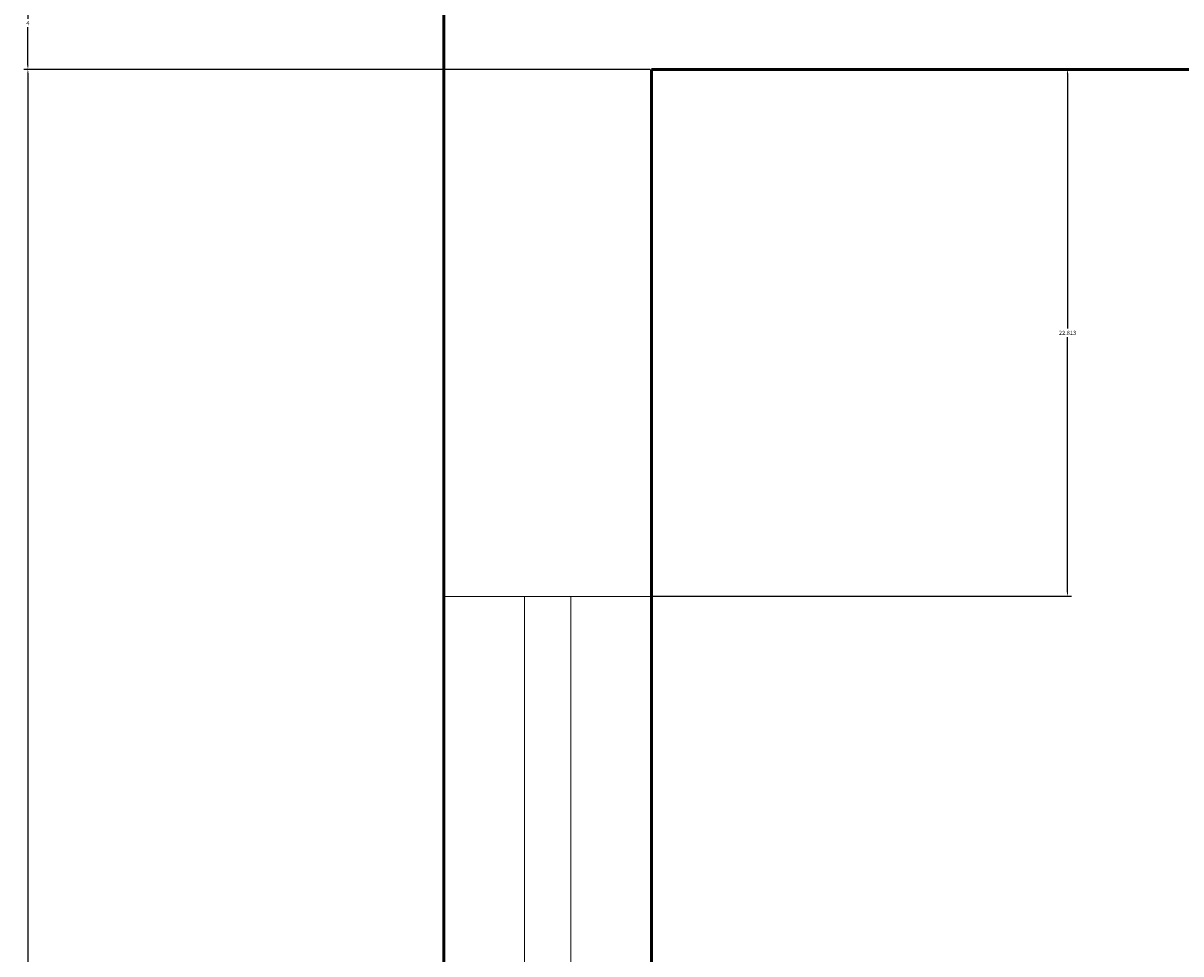
# Model space of a CAD drawing. Units: inches. Extents: x 2621 to 2849, y 2066 to 2463.
# Tile 9 of 28: x 2621 to 2671, y 2277 to 2317. Entities that reach past the tile are written whole.
import ezdxf

# ---------------------------------------------------------------- set-up
doc = ezdxf.new("R2010")
doc.units = ezdxf.units.IN
for name, color, linetype, lineweight in [('A-ANNO-DIMS', 2, 'Continuous', 18), ('A-GLAZ', 4, 'Continuous', 18), ('A-WALL', 7, 'Continuous', 50)]:
    doc.layers.add(name, color=color, linetype=linetype, lineweight=lineweight)
doc.styles.get("Standard").update_dxf_attribs({"font": 'arial.ttf'})
doc.dimstyles.get("Standard").update_dxf_attribs({"dimtxt": 0.18, "dimasz": 0.18, "dimexe": 0.18, "dimexo": 0.0625, "dimgap": 0.09, "dimtad": 0, "dimtih": 1, "dimtoh": 1, "dimdec": 4, "dimzin": 0, "dimdsep": 46, "dimtxsty": 'Standard', "dimcen": 0.09, "dimadec": 0, "dimazin": 0, "dimtfac": 1, "dimtdec": 4, "dimtofl": 0, "dimtmove": 0, "dimatfit": 3, "dimfxl": 1, "dimtolj": 1, "dimtzin": 0, "dimarcsym": 0})

# ---------------------------------------------------------------- blocks, each defined once
blk = doc.blocks.new('WIN-48IN')
for p, q in [((0, 5.5), (48, 5.5)), ((0, 3.5), (48, 3.5))]:
    blk.add_line(p, q)
blk.add_lwpolyline([(48, 9), (48, 0)])
blk = doc.blocks.new('*D44')
at = {"layer": 'A-ANNO-DIMS', "color": 0, "lineweight": -2, "transparency": 16777216}
for p, q in [((2647.933, 2315.375), (2666.054, 2315.375)), ((2665.874, 2315.195), (2665.874, 2304.15)), ((2665.874, 2292.742), (2665.874, 2303.786)), ((2647.933, 2292.562), (2666.054, 2292.562))]:
    blk.add_line(p, q, dxfattribs=at)
at = {"layer": 'A-ANNO-DIMS', "color": 0, "transparency": 16777216}
for points in [[(2665.844, 2315.195), (2665.904, 2315.195), (2665.874, 2315.375)], [(2665.844, 2292.742), (2665.904, 2292.742), (2665.874, 2292.562)]]:
    blk.add_solid(points, dxfattribs=at)
at = {"layer": 'Defpoints', "color": 0, "transparency": 16777216}
for p in [(2647.87, 2315.375), (2647.87, 2292.562), (2665.874, 2292.562)]:
    blk.add_point(p, dxfattribs=at)
at = {"layer": 'A-ANNO-DIMS', "color": 0, "transparency": 16777216, "insert": (2665.874, 2303.968), "char_height": 0.18, "attachment_point": 5}
blk.add_mtext('\\A1;22.813', dxfattribs=at)
blk = doc.blocks.new('*D49')
at = {"layer": 'A-ANNO-DIMS', "color": 0, "lineweight": -2, "transparency": 16777216}
for p, q in [((2647.807599, 2319.374587), (2620.686599, 2319.374587)), ((2620.866599, 2319.194587), (2620.866599, 2317.554587)), ((2620.866599, 2315.554587), (2620.866599, 2317.194587)), ((2647.807599, 2315.374587), (2620.686599, 2315.374587))]:
    blk.add_line(p, q, dxfattribs=at)
at = {"layer": 'A-ANNO-DIMS', "color": 0, "transparency": 16777216}
for points in [[(2620.836599, 2319.194587), (2620.896599, 2319.194587), (2620.866599, 2319.374587)], [(2620.836599, 2315.554587), (2620.896599, 2315.554587), (2620.866599, 2315.374587)]]:
    blk.add_solid(points, dxfattribs=at)
at = {"layer": 'Defpoints', "color": 0, "transparency": 16777216}
for p in [(2647.870099, 2319.374587), (2620.866599, 2315.374587), (2647.870099, 2315.374587)]:
    blk.add_point(p, dxfattribs=at)
at = {"layer": 'A-ANNO-DIMS', "color": 0, "transparency": 16777216, "insert": (2620.866599, 2317.374587), "char_height": 0.18, "attachment_point": 5}
blk.add_mtext('\\A1;4', dxfattribs=at)
blk = doc.blocks.new('*D57')
at = {"layer": 'A-ANNO-DIMS', "color": 0, "lineweight": -2, "transparency": 16777216}
for p, q in [((2647.808, 2315.375), (2620.687, 2315.375)), ((2620.867, 2315.195), (2620.867, 2257.556)), ((2620.867, 2199.555), (2620.867, 2257.193)), ((2647.808, 2199.375), (2620.687, 2199.375))]:
    blk.add_line(p, q, dxfattribs=at)
at = {"layer": 'A-ANNO-DIMS', "color": 0, "transparency": 16777216}
for points in [[(2620.837, 2315.195), (2620.897, 2315.195), (2620.867, 2315.375)], [(2620.837, 2199.555), (2620.897, 2199.555), (2620.867, 2199.375)]]:
    blk.add_solid(points, dxfattribs=at)
at = {"layer": 'Defpoints', "color": 0, "transparency": 16777216}
for p in [(2620.867, 2315.375), (2647.87, 2315.375), (2647.87, 2199.375)]:
    blk.add_point(p, dxfattribs=at)
at = {"layer": 'A-ANNO-DIMS', "color": 0, "transparency": 16777216, "insert": (2620.867, 2257.375), "char_height": 0.18, "attachment_point": 5}
blk.add_mtext('\\A1;116', dxfattribs=at)

msp = doc.modelspace()

# ---------------------------------------------------------------- linework, layer by layer
at = {"layer": 'A-WALL'}
for p, q in [((2647.8701, 2315.3746), (2763.8701, 2315.3746)), ((2647.8701, 2199.3746), (2647.8701, 2315.3746))]:
    msp.add_line(p, q, dxfattribs=at)
msp.add_lwpolyline([(2761.8701, 2084.3746), (2638.8701, 2084.3746), (2638.8701, 2444.3746), (2830.8701, 2444.3746), (2830.8701, 2084.3746), (2797.8701, 2084.3746)], dxfattribs=at)

# ---------------------------------------------------------------- block references
at = {"layer": 'A-GLAZ', "rotation": 90.00000000000018}
msp.add_blockref('WIN-48IN', (2647.8701, 2244.5617), dxfattribs=at)

# ---------------------------------------------------------------- dimensions: what is measured, and where the dimension line sits
at = {"layer": 'A-ANNO-DIMS'}
for base, p1, p2, angle, override, picture, middle in [((2620.8666, 2315.3746), (2647.8701, 2319.3746), (2647.8701, 2315.3746), 90, {"dimdec": 0, "dimlfac": 1, "dimrnd": 0, "dimzin": 0, "dimdsep": 46, "dimlunit": 2}, '*D49', (2620.8666, 2317.3746)), ((2620.8666, 2315.3746), (2647.8701, 2199.3746), (2647.8701, 2315.3746), 90, {"dimdec": 0, "dimlfac": 1, "dimrnd": 0, "dimzin": 0, "dimdsep": 46, "dimlunit": 2}, '*D57', (2620.8666, 2257.3746)), ((2665.8736, 2292.5617), (2647.8701, 2315.3746), (2647.8701, 2292.5617), 270, {"dimdec": 3, "dimlfac": 1, "dimrnd": 0, "dimzin": 0, "dimdsep": 46, "dimlunit": 2}, '*D44', (2665.8736, 2303.9682))]:
    dim = msp.add_linear_dim(base=base, p1=p1, p2=p2, angle=angle, dimstyle='Standard', override=override, dxfattribs=at)
    dim.commit()
    dim.dimension.update_dxf_attribs({"geometry": picture, "text_midpoint": middle})

doc.saveas('drawing.dxf')
